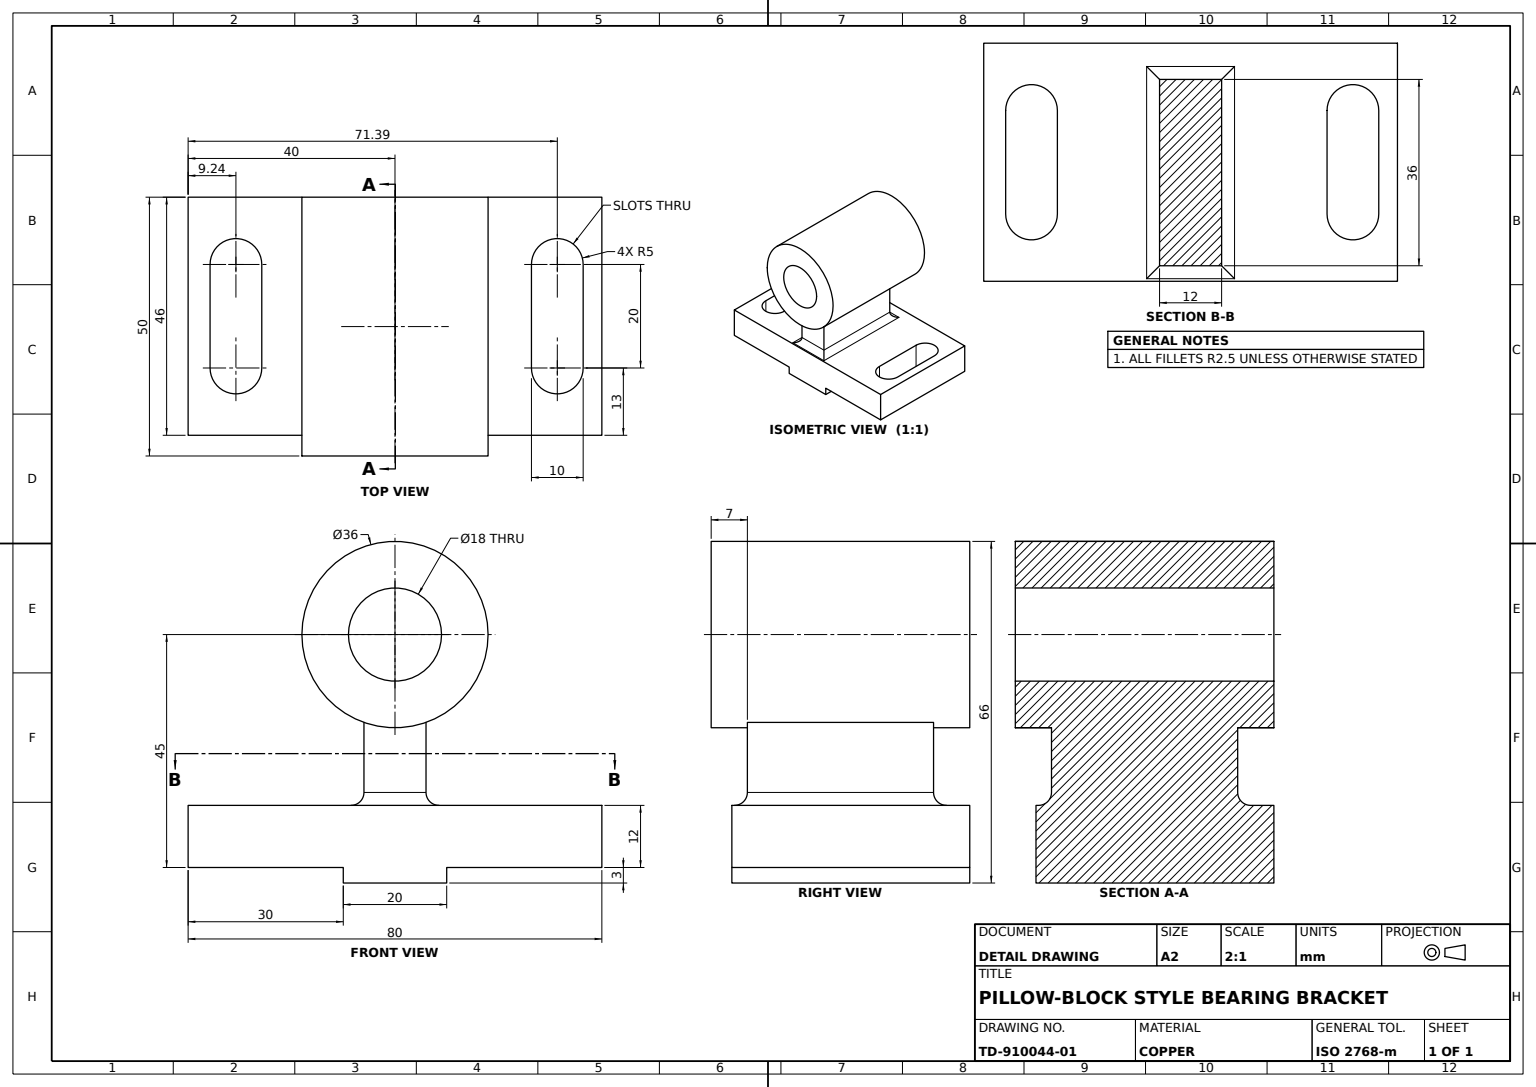
from build123d import *

# Parameters (mm, degrees)
BASE_PLATE_DEPTH             = 46
HUB_PROFILE_36_18_R          = 18
HUB_PROFILE_36_18_R_2        = 9
BEARING_HUB_36_BORE_18_DEPTH = 50
HUB_SUPPORT_WEB_REACH        = 109.243
HUB_SUPPORT_WEB_END_RADIUS   = 18
HUB_SUPPORT_PROFILE_W        = 36
HUB_SUPPORT_PROFILE_H        = 12
MOUNTING_SLOTS_2X_DEPTH      = 108.24271537
EDGE_FILLETS_R2_5_R          = 2.5


with BuildPart() as part:
    # Base Plate Profile → Base Plate (new body)
    with BuildSketch(Plane(origin=(0, 0, 0), x_dir=(0, 0, -1), z_dir=(1, 0, 0))):
        Polygon((0, 0), (30, 0), (30, -3), (50, -3), (50, 0), (80, 0), (80, 12), (0, 12), align=None)
    extrude(amount=BASE_PLATE_DEPTH)



with BuildPart() as body_2:
    # Hub Profile Ø36-Ø18 → Bearing Hub Ø36 Bore Ø18 (new body)
    with BuildSketch(Plane.ZY):
        with Locations((-40, 45)):
            Circle(HUB_PROFILE_36_18_R)
        with Locations((-40, 45)):
            Circle(HUB_PROFILE_36_18_R_2, mode=Mode.SUBTRACT)
    extrude(amount=-BEARING_HUB_36_BORE_18_DEPTH)


with BuildPart() as part_1:
    add(part.part)

    add(body_2.part)  # Hub Support Web merges body 2
    # Hub Support Web: up to this cylinder (the profile starts outside it)
    hub_support_web_end = Plane(origin=(25, 45, -40), z_dir=(-1, 0, 0)) * Cylinder(HUB_SUPPORT_WEB_END_RADIUS, 255.486, mode=Mode.PRIVATE)
    # Hub Support Profile → Hub Support Web (add, up to the surface)
    with BuildSketch(Plane(origin=(0, 12, 0), x_dir=(1, 0, 0), z_dir=(0, 1, 0)), mode=Mode.PRIVATE) as hub_support_web_sk1:
        with Locations((25, 40)):
            Rectangle(HUB_SUPPORT_PROFILE_W, HUB_SUPPORT_PROFILE_H)
    hub_support_web_tool1 = extrude(hub_support_web_sk1.sketch, amount=HUB_SUPPORT_WEB_REACH, mode=Mode.PRIVATE) - hub_support_web_end
    add(hub_support_web_tool1.solids().sort_by_distance((25, 12, -40))[0])

    # Mounting Slots Profile → Mounting Slots 2x (cut, through all)
    with BuildSketch(Plane(origin=(0, 12, 0), x_dir=(1, 0, 0), z_dir=(0, 1, 0))):
        with BuildLine():
            Line((13, 76.385225424), (33, 76.385225424))
            ThreePointArc((33, 76.385225424), (38, 71.385225424), (33, 66.385225424))
            Line((33, 66.385225424), (13, 66.385225424))
            ThreePointArc((13, 66.385225424), (8, 71.385225424), (13, 76.385225424))
        make_face()
        with BuildLine():
            Line((13, 14.243278019), (33, 14.243278019))
            ThreePointArc((33, 14.243278019), (38, 9.243278019), (33, 4.243278019))
            Line((33, 4.243278019), (13, 4.243278019))
            ThreePointArc((13, 4.243278019), (8, 9.243278019), (13, 14.243278019))
        make_face()
    extrude(amount=-MOUNTING_SLOTS_2X_DEPTH, mode=Mode.SUBTRACT)

    # Edge Fillets R2.5
    edge_fillets_r2_5_edges = [part_1.edges().sort_by_distance(p)[0] for p in [
        (25, 12, -34),
        (7, 12, -40),
        (25, 12, -46),
        (43, 12, -40),
    ]]
    fillet(edge_fillets_r2_5_edges, radius=EDGE_FILLETS_R2_5_R)


solid = part_1.part
